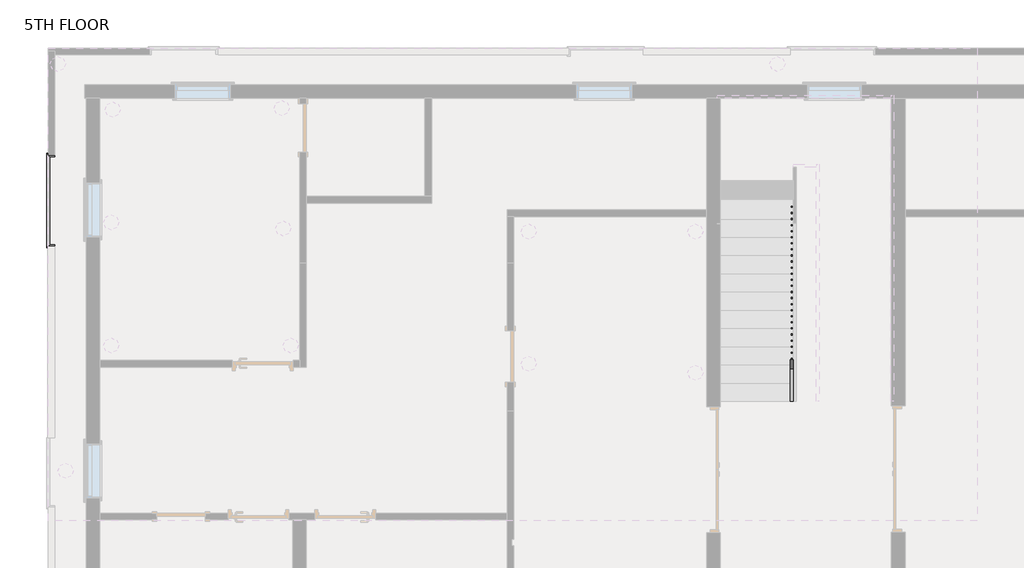
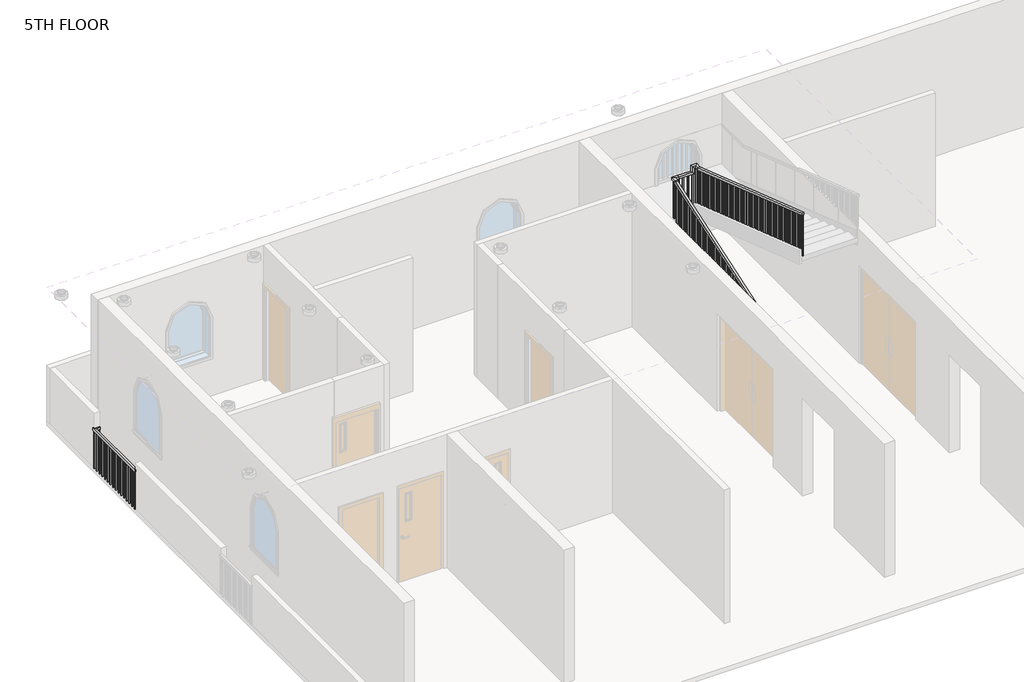
# One storey, part 4 of 7: 2 railings.
"""IFC4 building model written with IfcOpenShell, lengths in millimetres."""

from ifc_helpers import new_model, si_unit, frame, origin, place, context, project, spatial, polyline, outline, extrude, faceted_brep, element, save

model = new_model("IFC4")

# Units and contexts
model_context = context("Model", 3, world=origin())
ifc_project = project(units=[si_unit("LENGTHUNIT", "METRE", prefix="MILLI")], contexts=[model_context])

# Site, building, storey
site = spatial("IfcSite", under=ifc_project)
building = spatial("IfcBuilding", under=site)
storey = spatial("IfcBuildingStorey", under=building, Name="5TH FLOOR", Elevation=16002.0)

# Railings
placement = place(None, origin())
element("IfcRailing", 1, ObjectType="Handrail - Rectangular", at=placement, inside=storey, context=model_context, shape_type="SolidModel", body=[
    faceted_brep([(-680.3987998, 2564.5067329, 17019.8142857), (-680.3987998, 2564.5067329, 16966.1699957), (-629.5987998, 2564.5067329, 16966.1699957), (-629.5987998, 2564.5067329, 17019.8142857), (-680.3987998, 6450.7067329, 18338.3464286), (-680.3987998, 6501.5067329, 18301.9378529), (-629.5987998, 6501.5067329, 18301.9378529), (-629.5987998, 6450.7067329, 18338.3464286), (-553.3987998, 6577.7067329, 18313.4), (-553.3987998, 6577.7067329, 18364.2), (-273.9987915, 6577.7067329, 18364.2), (-223.1987915, 6577.7067329, 18313.4), (-553.3987998, 6526.9067329, 18313.4), (-223.1987915, 6526.9067329, 18313.4), (-553.3987998, 6526.9067329, 18364.2), (-273.9987915, 6526.9067329, 18364.2), (-146.9987915, 2564.5067329, 19812.0), (-197.7987915, 2564.5067329, 19812.0), (-197.7987915, 2564.5067329, 19758.35571), (-146.9987915, 2564.5067329, 19758.35571), (-146.9987915, 6442.3235624, 18442.6678571), (-146.9987915, 6450.7067329, 18493.4678571), (-197.7987915, 6442.3235624, 18442.6678571), (-197.7987915, 6450.7067329, 18493.4678571), (-680.3987998, 6450.7067329, 18364.2), (-680.3987998, 6501.5067329, 18313.4), (-629.5987998, 6501.5067329, 18313.4), (-629.5987998, 6450.7067329, 18364.2), (-680.3987998, 6577.7067329, 18364.2), (-680.3987998, 6577.7067329, 18313.4), (-629.5987998, 6526.9067329, 18313.4), (-629.5987998, 6526.9067329, 18364.2), (-273.9987915, 6577.7067329, 18493.4678571), (-223.1987915, 6577.7067329, 18442.6678571), (-223.1987915, 6526.9067329, 18442.6678571), (-273.9987915, 6526.9067329, 18493.4678571), (-146.9987915, 6577.7067329, 18493.4678571), (-146.9987915, 6577.7067329, 18442.6678571), (-197.7987915, 6526.9067329, 18442.6678571), (-197.7987915, 6526.9067329, 18493.4678571)], [[[0, 1, 2, 3]], [[1, 0, 4, 5]], [[2, 1, 5, 6]], [[3, 2, 6, 7]], [[0, 3, 7, 4]], [[8, 9, 10, 11]], [[12, 8, 11, 13]], [[14, 12, 13, 15]], [[9, 14, 15, 10]], [[16, 17, 18, 19]], [[20, 21, 16, 19]], [[22, 20, 19, 18]], [[23, 22, 18, 17]], [[21, 23, 17, 16]], [[5, 4, 24, 25]], [[6, 5, 25, 26]], [[7, 6, 26, 27]], [[4, 7, 27, 24]], [[25, 24, 28, 29]], [[26, 25, 29, 30]], [[27, 26, 30, 31]], [[24, 27, 31, 28]], [[29, 28, 9, 8]], [[30, 29, 8, 12]], [[31, 30, 12, 14]], [[28, 31, 14, 9]], [[11, 10, 32, 33]], [[13, 11, 33, 34]], [[15, 13, 34, 35]], [[10, 15, 35, 32]], [[33, 32, 36, 37]], [[34, 33, 37, 38]], [[35, 34, 38, 39]], [[32, 35, 39, 36]], [[37, 36, 21, 20]], [[38, 37, 20, 22]], [[39, 38, 22, 23]], [[36, 39, 23, 21]]]),
    extrude(outline(polyline([(2580.3817329, 19752.9695493), (2599.4317329, 19746.5061565), (2599.4317329, 18794.1857143), (2580.3817329, 18794.1857143), (2580.3817329, 19752.9695493)])), frame((-181.9237915, 0.0, 0.0), z_axis=(1.0, 0.0, 0.0), x_axis=(0.0, 1.0, 0.0)), (0.0, 0.0, 1.0), 19.05),
    extrude(outline(polyline([(2681.9817329, 19718.4981207), (2701.0317329, 19712.0347279), (2701.0317329, 18794.1857143), (2681.9817329, 18794.1857143), (2681.9817329, 19718.4981207)])), frame((-181.9237915, 0.0, 0.0), z_axis=(1.0, 0.0, 0.0), x_axis=(0.0, 1.0, 0.0)), (0.0, 0.0, 1.0), 19.05),
    extrude(outline(polyline([(2783.5817329, 19684.0266922), (2802.6317329, 19677.5632993), (2802.6317329, 18794.1857143), (2783.5817329, 18794.1857143), (2783.5817329, 19684.0266922)])), frame((-181.9237915, 0.0, 0.0), z_axis=(1.0, 0.0, 0.0), x_axis=(0.0, 1.0, 0.0)), (0.0, 0.0, 1.0), 19.05),
    extrude(outline(polyline([(2885.1817329, 19649.5552636), (2904.2317329, 19643.0918707), (2904.2317329, 18690.7714286), (2885.1817329, 18690.7714286), (2885.1817329, 19649.5552636)])), frame((-181.9237915, 0.0, 0.0), z_axis=(1.0, 0.0, 0.0), x_axis=(0.0, 1.0, 0.0)), (0.0, 0.0, 1.0), 19.05),
    extrude(outline(polyline([(2986.7817329, 19615.083835), (3005.8317329, 19608.6204422), (3005.8317329, 18690.7714286), (2986.7817329, 18690.7714286), (2986.7817329, 19615.083835)])), frame((-181.9237915, 0.0, 0.0), z_axis=(1.0, 0.0, 0.0), x_axis=(0.0, 1.0, 0.0)), (0.0, 0.0, 1.0), 19.05),
    extrude(outline(polyline([(3088.3817329, 19580.6124065), (3107.4317329, 19574.1490136), (3107.4317329, 18690.7714286), (3088.3817329, 18690.7714286), (3088.3817329, 19580.6124065)])), frame((-181.9237915, 0.0, 0.0), z_axis=(1.0, 0.0, 0.0), x_axis=(0.0, 1.0, 0.0)), (0.0, 0.0, 1.0), 19.05),
    extrude(outline(polyline([(3189.9817329, 19546.1409779), (3209.0317329, 19539.677585), (3209.0317329, 18587.3571429), (3189.9817329, 18587.3571429), (3189.9817329, 19546.1409779)])), frame((-181.9237915, 0.0, 0.0), z_axis=(1.0, 0.0, 0.0), x_axis=(0.0, 1.0, 0.0)), (0.0, 0.0, 1.0), 19.05),
    extrude(outline(polyline([(3291.5817329, 19511.6695493), (3310.6317329, 19505.2061565), (3310.6317329, 18587.3571429), (3291.5817329, 18587.3571429), (3291.5817329, 19511.6695493)])), frame((-181.9237915, 0.0, 0.0), z_axis=(1.0, 0.0, 0.0), x_axis=(0.0, 1.0, 0.0)), (0.0, 0.0, 1.0), 19.05),
    extrude(outline(polyline([(3393.1817329, 19477.1981207), (3412.2317329, 19470.7347279), (3412.2317329, 18587.3571429), (3393.1817329, 18587.3571429), (3393.1817329, 19477.1981207)])), frame((-181.9237915, 0.0, 0.0), z_axis=(1.0, 0.0, 0.0), x_axis=(0.0, 1.0, 0.0)), (0.0, 0.0, 1.0), 19.05),
    extrude(outline(polyline([(3494.7817329, 19442.7266922), (3513.8317329, 19436.2632993), (3513.8317329, 18483.9428571), (3494.7817329, 18483.9428571), (3494.7817329, 19442.7266922)])), frame((-181.9237915, 0.0, 0.0), z_axis=(1.0, 0.0, 0.0), x_axis=(0.0, 1.0, 0.0)), (0.0, 0.0, 1.0), 19.05),
    extrude(outline(polyline([(3596.3817329, 19408.2552636), (3615.4317329, 19401.7918707), (3615.4317329, 18483.9428571), (3596.3817329, 18483.9428571), (3596.3817329, 19408.2552636)])), frame((-181.9237915, 0.0, 0.0), z_axis=(1.0, 0.0, 0.0), x_axis=(0.0, 1.0, 0.0)), (0.0, 0.0, 1.0), 19.05),
    extrude(outline(polyline([(3697.9817329, 19373.783835), (3717.0317329, 19367.3204422), (3717.0317329, 18483.9428571), (3697.9817329, 18483.9428571), (3697.9817329, 19373.783835)])), frame((-181.9237915, 0.0, 0.0), z_axis=(1.0, 0.0, 0.0), x_axis=(0.0, 1.0, 0.0)), (0.0, 0.0, 1.0), 19.05),
    extrude(outline(polyline([(3799.5817329, 19339.3124065), (3818.6317329, 19332.8490136), (3818.6317329, 18380.5285714), (3799.5817329, 18380.5285714), (3799.5817329, 19339.3124065)])), frame((-181.9237915, 0.0, 0.0), z_axis=(1.0, 0.0, 0.0), x_axis=(0.0, 1.0, 0.0)), (0.0, 0.0, 1.0), 19.05),
    extrude(outline(polyline([(3901.1817329, 19304.8409779), (3920.2317329, 19298.377585), (3920.2317329, 18380.5285714), (3901.1817329, 18380.5285714), (3901.1817329, 19304.8409779)])), frame((-181.9237915, 0.0, 0.0), z_axis=(1.0, 0.0, 0.0), x_axis=(0.0, 1.0, 0.0)), (0.0, 0.0, 1.0), 19.05),
    extrude(outline(polyline([(4002.7817329, 19270.3695493), (4021.8317329, 19263.9061565), (4021.8317329, 18380.5285714), (4002.7817329, 18380.5285714), (4002.7817329, 19270.3695493)])), frame((-181.9237915, 0.0, 0.0), z_axis=(1.0, 0.0, 0.0), x_axis=(0.0, 1.0, 0.0)), (0.0, 0.0, 1.0), 19.05),
    extrude(outline(polyline([(4104.3817329, 19235.8981207), (4123.4317329, 19229.4347279), (4123.4317329, 18277.1142857), (4104.3817329, 18277.1142857), (4104.3817329, 19235.8981207)])), frame((-181.9237915, 0.0, 0.0), z_axis=(1.0, 0.0, 0.0), x_axis=(0.0, 1.0, 0.0)), (0.0, 0.0, 1.0), 19.05),
    extrude(outline(polyline([(4205.9817329, 19201.4266922), (4225.0317329, 19194.9632993), (4225.0317329, 18277.1142857), (4205.9817329, 18277.1142857), (4205.9817329, 19201.4266922)])), frame((-181.9237915, 0.0, 0.0), z_axis=(1.0, 0.0, 0.0), x_axis=(0.0, 1.0, 0.0)), (0.0, 0.0, 1.0), 19.05),
    extrude(outline(polyline([(4307.5817329, 19166.9552636), (4326.6317329, 19160.4918707), (4326.6317329, 18277.1142857), (4307.5817329, 18277.1142857), (4307.5817329, 19166.9552636)])), frame((-181.9237915, 0.0, 0.0), z_axis=(1.0, 0.0, 0.0), x_axis=(0.0, 1.0, 0.0)), (0.0, 0.0, 1.0), 19.05),
    extrude(outline(polyline([(4409.1817329, 19132.483835), (4428.2317329, 19126.0204422), (4428.2317329, 18173.7), (4409.1817329, 18173.7), (4409.1817329, 19132.483835)])), frame((-181.9237915, 0.0, 0.0), z_axis=(1.0, 0.0, 0.0), x_axis=(0.0, 1.0, 0.0)), (0.0, 0.0, 1.0), 19.05),
    extrude(outline(polyline([(4510.7817329, 19098.0124065), (4529.8317329, 19091.5490136), (4529.8317329, 18173.7), (4510.7817329, 18173.7), (4510.7817329, 19098.0124065)])), frame((-181.9237915, 0.0, 0.0), z_axis=(1.0, 0.0, 0.0), x_axis=(0.0, 1.0, 0.0)), (0.0, 0.0, 1.0), 19.05),
    extrude(outline(polyline([(4612.3817329, 19063.5409779), (4631.4317329, 19057.077585), (4631.4317329, 18173.7), (4612.3817329, 18173.7), (4612.3817329, 19063.5409779)])), frame((-181.9237915, 0.0, 0.0), z_axis=(1.0, 0.0, 0.0), x_axis=(0.0, 1.0, 0.0)), (0.0, 0.0, 1.0), 19.05),
    extrude(outline(polyline([(4713.9817329, 19029.0695493), (4733.0317329, 19022.6061565), (4733.0317329, 18070.2857143), (4713.9817329, 18070.2857143), (4713.9817329, 19029.0695493)])), frame((-181.9237915, 0.0, 0.0), z_axis=(1.0, 0.0, 0.0), x_axis=(0.0, 1.0, 0.0)), (0.0, 0.0, 1.0), 19.05),
    extrude(outline(polyline([(4815.5817329, 18994.5981207), (4834.6317329, 18988.1347279), (4834.6317329, 18070.2857143), (4815.5817329, 18070.2857143), (4815.5817329, 18994.5981207)])), frame((-181.9237915, 0.0, 0.0), z_axis=(1.0, 0.0, 0.0), x_axis=(0.0, 1.0, 0.0)), (0.0, 0.0, 1.0), 19.05),
    extrude(outline(polyline([(4917.1817329, 18960.1266922), (4936.2317329, 18953.6632993), (4936.2317329, 18070.2857143), (4917.1817329, 18070.2857143), (4917.1817329, 18960.1266922)])), frame((-181.9237915, 0.0, 0.0), z_axis=(1.0, 0.0, 0.0), x_axis=(0.0, 1.0, 0.0)), (0.0, 0.0, 1.0), 19.05),
    extrude(outline(polyline([(5018.7817329, 18925.6552636), (5037.8317329, 18919.1918707), (5037.8317329, 17966.8714286), (5018.7817329, 17966.8714286), (5018.7817329, 18925.6552636)])), frame((-181.9237915, 0.0, 0.0), z_axis=(1.0, 0.0, 0.0), x_axis=(0.0, 1.0, 0.0)), (0.0, 0.0, 1.0), 19.05),
    extrude(outline(polyline([(5120.3817329, 18891.183835), (5139.4317329, 18884.7204422), (5139.4317329, 17966.8714286), (5120.3817329, 17966.8714286), (5120.3817329, 18891.183835)])), frame((-181.9237915, 0.0, 0.0), z_axis=(1.0, 0.0, 0.0), x_axis=(0.0, 1.0, 0.0)), (0.0, 0.0, 1.0), 19.05),
    extrude(outline(polyline([(5221.9817329, 18856.7124065), (5241.0317329, 18850.2490136), (5241.0317329, 17966.8714286), (5221.9817329, 17966.8714286), (5221.9817329, 18856.7124065)])), frame((-181.9237915, 0.0, 0.0), z_axis=(1.0, 0.0, 0.0), x_axis=(0.0, 1.0, 0.0)), (0.0, 0.0, 1.0), 19.05),
    extrude(outline(polyline([(5323.5817329, 18822.2409779), (5342.6317329, 18815.777585), (5342.6317329, 17863.4571429), (5323.5817329, 17863.4571429), (5323.5817329, 18822.2409779)])), frame((-181.9237915, 0.0, 0.0), z_axis=(1.0, 0.0, 0.0), x_axis=(0.0, 1.0, 0.0)), (0.0, 0.0, 1.0), 19.05),
    extrude(outline(polyline([(5425.1817329, 18787.7695493), (5444.2317329, 18781.3061565), (5444.2317329, 17863.4571429), (5425.1817329, 17863.4571429), (5425.1817329, 18787.7695493)])), frame((-181.9237915, 0.0, 0.0), z_axis=(1.0, 0.0, 0.0), x_axis=(0.0, 1.0, 0.0)), (0.0, 0.0, 1.0), 19.05),
    extrude(outline(polyline([(5526.7817329, 18753.2981207), (5545.8317329, 18746.8347279), (5545.8317329, 17863.4571429), (5526.7817329, 17863.4571429), (5526.7817329, 18753.2981207)])), frame((-181.9237915, 0.0, 0.0), z_axis=(1.0, 0.0, 0.0), x_axis=(0.0, 1.0, 0.0)), (0.0, 0.0, 1.0), 19.05),
    extrude(outline(polyline([(5628.3817329, 18718.8266922), (5647.4317329, 18712.3632993), (5647.4317329, 17760.0428571), (5628.3817329, 17760.0428571), (5628.3817329, 18718.8266922)])), frame((-181.9237915, 0.0, 0.0), z_axis=(1.0, 0.0, 0.0), x_axis=(0.0, 1.0, 0.0)), (0.0, 0.0, 1.0), 19.05),
    extrude(outline(polyline([(5729.9817329, 18684.3552636), (5749.0317329, 18677.8918707), (5749.0317329, 17760.0428571), (5729.9817329, 17760.0428571), (5729.9817329, 18684.3552636)])), frame((-181.9237915, 0.0, 0.0), z_axis=(1.0, 0.0, 0.0), x_axis=(0.0, 1.0, 0.0)), (0.0, 0.0, 1.0), 19.05),
    extrude(outline(polyline([(5831.5817329, 18649.883835), (5850.6317329, 18643.4204422), (5850.6317329, 17760.0428571), (5831.5817329, 17760.0428571), (5831.5817329, 18649.883835)])), frame((-181.9237915, 0.0, 0.0), z_axis=(1.0, 0.0, 0.0), x_axis=(0.0, 1.0, 0.0)), (0.0, 0.0, 1.0), 19.05),
    extrude(outline(polyline([(5933.1817329, 18615.4124065), (5952.2317329, 18608.9490136), (5952.2317329, 17656.6285714), (5933.1817329, 17656.6285714), (5933.1817329, 18615.4124065)])), frame((-181.9237915, 0.0, 0.0), z_axis=(1.0, 0.0, 0.0), x_axis=(0.0, 1.0, 0.0)), (0.0, 0.0, 1.0), 19.05),
    extrude(outline(polyline([(6034.7817329, 18580.9409779), (6053.8317329, 18574.477585), (6053.8317329, 17656.6285714), (6034.7817329, 17656.6285714), (6034.7817329, 18580.9409779)])), frame((-181.9237915, 0.0, 0.0), z_axis=(1.0, 0.0, 0.0), x_axis=(0.0, 1.0, 0.0)), (0.0, 0.0, 1.0), 19.05),
    extrude(outline(polyline([(6136.3817329, 18546.4695493), (6155.4317329, 18540.0061565), (6155.4317329, 17656.6285714), (6136.3817329, 17656.6285714), (6136.3817329, 18546.4695493)])), frame((-181.9237915, 0.0, 0.0), z_axis=(1.0, 0.0, 0.0), x_axis=(0.0, 1.0, 0.0)), (0.0, 0.0, 1.0), 19.05),
    extrude(outline(polyline([(6237.9817329, 18511.9981207), (6257.0317329, 18505.5347279), (6257.0317329, 17553.2142857), (6237.9817329, 17553.2142857), (6237.9817329, 18511.9981207)])), frame((-181.9237915, 0.0, 0.0), z_axis=(1.0, 0.0, 0.0), x_axis=(0.0, 1.0, 0.0)), (0.0, 0.0, 1.0), 19.05),
    extrude(outline(polyline([(6339.5817329, 18477.5266922), (6358.6317329, 18471.0632993), (6358.6317329, 17553.2142857), (6339.5817329, 17553.2142857), (6339.5817329, 18477.5266922)])), frame((-181.9237915, 0.0, 0.0), z_axis=(1.0, 0.0, 0.0), x_axis=(0.0, 1.0, 0.0)), (0.0, 0.0, 1.0), 19.05),
    extrude(outline(polyline([(6441.1817329, 18443.0552636), (6460.2317329, 18436.5918707), (6460.2317329, 17553.2142857), (6441.1817329, 17553.2142857), (6441.1817329, 18443.0552636)])), frame((-181.9237915, 0.0, 0.0), z_axis=(1.0, 0.0, 0.0), x_axis=(0.0, 1.0, 0.0)), (0.0, 0.0, 1.0), 19.05),
    extrude(outline(polyline([(-258.1237998, 6542.7817329), (-258.1237998, 6561.8317329), (-239.0737998, 6561.8317329), (-239.0737998, 6542.7817329), (-258.1237998, 6542.7817329)])), frame((0.0, 0.0, 17449.8), z_axis=(0.0, 0.0, 1.0), x_axis=(1.0, 0.0, 0.0)), (0.0, 0.0, 1.0), 992.8678571),
    extrude(outline(polyline([(-359.7237998, 6542.7817329), (-359.7237998, 6561.8317329), (-340.6737998, 6561.8317329), (-340.6737998, 6542.7817329), (-359.7237998, 6542.7817329)])), frame((0.0, 0.0, 17449.8), z_axis=(0.0, 0.0, 1.0), x_axis=(1.0, 0.0, 0.0)), (0.0, 0.0, 1.0), 863.6),
    extrude(outline(polyline([(-461.3237998, 6542.7817329), (-461.3237998, 6561.8317329), (-442.2737998, 6561.8317329), (-442.2737998, 6542.7817329), (-461.3237998, 6542.7817329)])), frame((0.0, 0.0, 17449.8), z_axis=(0.0, 0.0, 1.0), x_axis=(1.0, 0.0, 0.0)), (0.0, 0.0, 1.0), 863.6),
    extrude(outline(polyline([(-562.9237998, 6542.7817329), (-562.9237998, 6561.8317329), (-543.8737998, 6561.8317329), (-543.8737998, 6542.7817329), (-562.9237998, 6542.7817329)])), frame((0.0, 0.0, 17449.8), z_axis=(0.0, 0.0, 1.0), x_axis=(1.0, 0.0, 0.0)), (0.0, 0.0, 1.0), 863.6),
    extrude(outline(polyline([(-645.4737998, 6517.3817329), (-664.5237998, 6517.3817329), (-664.5237998, 6536.4317329), (-645.4737998, 6536.4317329), (-645.4737998, 6517.3817329)])), frame((0.0, 0.0, 17449.8), z_axis=(0.0, 0.0, 1.0), x_axis=(1.0, 0.0, 0.0)), (0.0, 0.0, 1.0), 863.6),
    extrude(outline(polyline([(6415.7817329, 18272.852585), (6434.8317329, 18279.3159779), (6434.8317329, 17346.3857143), (6415.7817329, 17346.3857143), (6415.7817329, 18272.852585)])), frame((-664.5237998, 0.0, 0.0), z_axis=(1.0, 0.0, 0.0), x_axis=(0.0, 1.0, 0.0)), (0.0, 0.0, 1.0), 19.05),
    extrude(outline(polyline([(6314.1817329, 18238.3811565), (6333.2317329, 18244.8445493), (6333.2317329, 17346.3857143), (6314.1817329, 17346.3857143), (6314.1817329, 18238.3811565)])), frame((-664.5237998, 0.0, 0.0), z_axis=(1.0, 0.0, 0.0), x_axis=(0.0, 1.0, 0.0)), (0.0, 0.0, 1.0), 19.05),
    extrude(outline(polyline([(6212.5817329, 18203.9097279), (6231.6317329, 18210.3731207), (6231.6317329, 17346.3857143), (6212.5817329, 17346.3857143), (6212.5817329, 18203.9097279)])), frame((-664.5237998, 0.0, 0.0), z_axis=(1.0, 0.0, 0.0), x_axis=(0.0, 1.0, 0.0)), (0.0, 0.0, 1.0), 19.05),
    extrude(outline(polyline([(6110.9817329, 18169.4382993), (6130.0317329, 18175.9016922), (6130.0317329, 17242.9714286), (6110.9817329, 17242.9714286), (6110.9817329, 18169.4382993)])), frame((-664.5237998, 0.0, 0.0), z_axis=(1.0, 0.0, 0.0), x_axis=(0.0, 1.0, 0.0)), (0.0, 0.0, 1.0), 19.05),
    extrude(outline(polyline([(6009.3817329, 18134.9668707), (6028.4317329, 18141.4302636), (6028.4317329, 17242.9714286), (6009.3817329, 17242.9714286), (6009.3817329, 18134.9668707)])), frame((-664.5237998, 0.0, 0.0), z_axis=(1.0, 0.0, 0.0), x_axis=(0.0, 1.0, 0.0)), (0.0, 0.0, 1.0), 19.05),
    extrude(outline(polyline([(5907.7817329, 18100.4954422), (5926.8317329, 18106.958835), (5926.8317329, 17242.9714286), (5907.7817329, 17242.9714286), (5907.7817329, 18100.4954422)])), frame((-664.5237998, 0.0, 0.0), z_axis=(1.0, 0.0, 0.0), x_axis=(0.0, 1.0, 0.0)), (0.0, 0.0, 1.0), 19.05),
    extrude(outline(polyline([(5806.1817329, 18066.0240136), (5825.2317329, 18072.4874065), (5825.2317329, 17139.5571429), (5806.1817329, 17139.5571429), (5806.1817329, 18066.0240136)])), frame((-664.5237998, 0.0, 0.0), z_axis=(1.0, 0.0, 0.0), x_axis=(0.0, 1.0, 0.0)), (0.0, 0.0, 1.0), 19.05),
    extrude(outline(polyline([(5704.5817329, 18031.552585), (5723.6317329, 18038.0159779), (5723.6317329, 17139.5571429), (5704.5817329, 17139.5571429), (5704.5817329, 18031.552585)])), frame((-664.5237998, 0.0, 0.0), z_axis=(1.0, 0.0, 0.0), x_axis=(0.0, 1.0, 0.0)), (0.0, 0.0, 1.0), 19.05),
    extrude(outline(polyline([(5602.9817329, 17997.0811565), (5622.0317329, 18003.5445493), (5622.0317329, 17139.5571429), (5602.9817329, 17139.5571429), (5602.9817329, 17997.0811565)])), frame((-664.5237998, 0.0, 0.0), z_axis=(1.0, 0.0, 0.0), x_axis=(0.0, 1.0, 0.0)), (0.0, 0.0, 1.0), 19.05),
    extrude(outline(polyline([(5501.3817329, 17962.6097279), (5520.4317329, 17969.0731207), (5520.4317329, 17036.1428571), (5501.3817329, 17036.1428571), (5501.3817329, 17962.6097279)])), frame((-664.5237998, 0.0, 0.0), z_axis=(1.0, 0.0, 0.0), x_axis=(0.0, 1.0, 0.0)), (0.0, 0.0, 1.0), 19.05),
    extrude(outline(polyline([(5399.7817329, 17928.1382993), (5418.8317329, 17934.6016922), (5418.8317329, 17036.1428571), (5399.7817329, 17036.1428571), (5399.7817329, 17928.1382993)])), frame((-664.5237998, 0.0, 0.0), z_axis=(1.0, 0.0, 0.0), x_axis=(0.0, 1.0, 0.0)), (0.0, 0.0, 1.0), 19.05),
    extrude(outline(polyline([(5298.1817329, 17893.6668707), (5317.2317329, 17900.1302636), (5317.2317329, 17036.1428571), (5298.1817329, 17036.1428571), (5298.1817329, 17893.6668707)])), frame((-664.5237998, 0.0, 0.0), z_axis=(1.0, 0.0, 0.0), x_axis=(0.0, 1.0, 0.0)), (0.0, 0.0, 1.0), 19.05),
    extrude(outline(polyline([(5196.5817329, 17859.1954422), (5215.6317329, 17865.658835), (5215.6317329, 16932.7285714), (5196.5817329, 16932.7285714), (5196.5817329, 17859.1954422)])), frame((-664.5237998, 0.0, 0.0), z_axis=(1.0, 0.0, 0.0), x_axis=(0.0, 1.0, 0.0)), (0.0, 0.0, 1.0), 19.05),
    extrude(outline(polyline([(5094.9817329, 17824.7240136), (5114.0317329, 17831.1874065), (5114.0317329, 16932.7285714), (5094.9817329, 16932.7285714), (5094.9817329, 17824.7240136)])), frame((-664.5237998, 0.0, 0.0), z_axis=(1.0, 0.0, 0.0), x_axis=(0.0, 1.0, 0.0)), (0.0, 0.0, 1.0), 19.05),
    extrude(outline(polyline([(4993.3817329, 17790.252585), (5012.4317329, 17796.7159779), (5012.4317329, 16932.7285714), (4993.3817329, 16932.7285714), (4993.3817329, 17790.252585)])), frame((-664.5237998, 0.0, 0.0), z_axis=(1.0, 0.0, 0.0), x_axis=(0.0, 1.0, 0.0)), (0.0, 0.0, 1.0), 19.05),
    extrude(outline(polyline([(4891.7817329, 17755.7811565), (4910.8317329, 17762.2445493), (4910.8317329, 16829.3142857), (4891.7817329, 16829.3142857), (4891.7817329, 17755.7811565)])), frame((-664.5237998, 0.0, 0.0), z_axis=(1.0, 0.0, 0.0), x_axis=(0.0, 1.0, 0.0)), (0.0, 0.0, 1.0), 19.05),
    extrude(outline(polyline([(4790.1817329, 17721.3097279), (4809.2317329, 17727.7731207), (4809.2317329, 16829.3142857), (4790.1817329, 16829.3142857), (4790.1817329, 17721.3097279)])), frame((-664.5237998, 0.0, 0.0), z_axis=(1.0, 0.0, 0.0), x_axis=(0.0, 1.0, 0.0)), (0.0, 0.0, 1.0), 19.05),
    extrude(outline(polyline([(4688.5817329, 17686.8382993), (4707.6317329, 17693.3016922), (4707.6317329, 16829.3142857), (4688.5817329, 16829.3142857), (4688.5817329, 17686.8382993)])), frame((-664.5237998, 0.0, 0.0), z_axis=(1.0, 0.0, 0.0), x_axis=(0.0, 1.0, 0.0)), (0.0, 0.0, 1.0), 19.05),
    extrude(outline(polyline([(4586.9817329, 17652.3668707), (4606.0317329, 17658.8302636), (4606.0317329, 16725.9), (4586.9817329, 16725.9), (4586.9817329, 17652.3668707)])), frame((-664.5237998, 0.0, 0.0), z_axis=(1.0, 0.0, 0.0), x_axis=(0.0, 1.0, 0.0)), (0.0, 0.0, 1.0), 19.05),
    extrude(outline(polyline([(4485.3817329, 17617.8954422), (4504.4317329, 17624.358835), (4504.4317329, 16725.9), (4485.3817329, 16725.9), (4485.3817329, 17617.8954422)])), frame((-664.5237998, 0.0, 0.0), z_axis=(1.0, 0.0, 0.0), x_axis=(0.0, 1.0, 0.0)), (0.0, 0.0, 1.0), 19.05),
    extrude(outline(polyline([(4383.7817329, 17583.4240136), (4402.8317329, 17589.8874065), (4402.8317329, 16725.9), (4383.7817329, 16725.9), (4383.7817329, 17583.4240136)])), frame((-664.5237998, 0.0, 0.0), z_axis=(1.0, 0.0, 0.0), x_axis=(0.0, 1.0, 0.0)), (0.0, 0.0, 1.0), 19.05),
    extrude(outline(polyline([(4282.1817329, 17548.952585), (4301.2317329, 17555.4159779), (4301.2317329, 16622.4857143), (4282.1817329, 16622.4857143), (4282.1817329, 17548.952585)])), frame((-664.5237998, 0.0, 0.0), z_axis=(1.0, 0.0, 0.0), x_axis=(0.0, 1.0, 0.0)), (0.0, 0.0, 1.0), 19.05),
    extrude(outline(polyline([(4180.5817329, 17514.4811565), (4199.6317329, 17520.9445493), (4199.6317329, 16622.4857143), (4180.5817329, 16622.4857143), (4180.5817329, 17514.4811565)])), frame((-664.5237998, 0.0, 0.0), z_axis=(1.0, 0.0, 0.0), x_axis=(0.0, 1.0, 0.0)), (0.0, 0.0, 1.0), 19.05),
    extrude(outline(polyline([(4078.9817329, 17480.0097279), (4098.0317329, 17486.4731207), (4098.0317329, 16622.4857143), (4078.9817329, 16622.4857143), (4078.9817329, 17480.0097279)])), frame((-664.5237998, 0.0, 0.0), z_axis=(1.0, 0.0, 0.0), x_axis=(0.0, 1.0, 0.0)), (0.0, 0.0, 1.0), 19.05),
    extrude(outline(polyline([(3977.3817329, 17445.5382993), (3996.4317329, 17452.0016922), (3996.4317329, 16519.0714286), (3977.3817329, 16519.0714286), (3977.3817329, 17445.5382993)])), frame((-664.5237998, 0.0, 0.0), z_axis=(1.0, 0.0, 0.0), x_axis=(0.0, 1.0, 0.0)), (0.0, 0.0, 1.0), 19.05),
    extrude(outline(polyline([(3875.7817329, 17411.0668707), (3894.8317329, 17417.5302636), (3894.8317329, 16519.0714286), (3875.7817329, 16519.0714286), (3875.7817329, 17411.0668707)])), frame((-664.5237998, 0.0, 0.0), z_axis=(1.0, 0.0, 0.0), x_axis=(0.0, 1.0, 0.0)), (0.0, 0.0, 1.0), 19.05),
    extrude(outline(polyline([(3774.1817329, 17376.5954422), (3793.2317329, 17383.058835), (3793.2317329, 16519.0714286), (3774.1817329, 16519.0714286), (3774.1817329, 17376.5954422)])), frame((-664.5237998, 0.0, 0.0), z_axis=(1.0, 0.0, 0.0), x_axis=(0.0, 1.0, 0.0)), (0.0, 0.0, 1.0), 19.05),
    extrude(outline(polyline([(3672.5817329, 17342.1240136), (3691.6317329, 17348.5874065), (3691.6317329, 16415.6571429), (3672.5817329, 16415.6571429), (3672.5817329, 17342.1240136)])), frame((-664.5237998, 0.0, 0.0), z_axis=(1.0, 0.0, 0.0), x_axis=(0.0, 1.0, 0.0)), (0.0, 0.0, 1.0), 19.05),
    extrude(outline(polyline([(3570.9817329, 17307.652585), (3590.0317329, 17314.1159779), (3590.0317329, 16415.6571429), (3570.9817329, 16415.6571429), (3570.9817329, 17307.652585)])), frame((-664.5237998, 0.0, 0.0), z_axis=(1.0, 0.0, 0.0), x_axis=(0.0, 1.0, 0.0)), (0.0, 0.0, 1.0), 19.05),
    extrude(outline(polyline([(3469.3817329, 17273.1811565), (3488.4317329, 17279.6445493), (3488.4317329, 16415.6571429), (3469.3817329, 16415.6571429), (3469.3817329, 17273.1811565)])), frame((-664.5237998, 0.0, 0.0), z_axis=(1.0, 0.0, 0.0), x_axis=(0.0, 1.0, 0.0)), (0.0, 0.0, 1.0), 19.05),
    extrude(outline(polyline([(3367.7817329, 17238.7097279), (3386.8317329, 17245.1731207), (3386.8317329, 16312.2428571), (3367.7817329, 16312.2428571), (3367.7817329, 17238.7097279)])), frame((-664.5237998, 0.0, 0.0), z_axis=(1.0, 0.0, 0.0), x_axis=(0.0, 1.0, 0.0)), (0.0, 0.0, 1.0), 19.05),
    extrude(outline(polyline([(3266.1817329, 17204.2382993), (3285.2317329, 17210.7016922), (3285.2317329, 16312.2428571), (3266.1817329, 16312.2428571), (3266.1817329, 17204.2382993)])), frame((-664.5237998, 0.0, 0.0), z_axis=(1.0, 0.0, 0.0), x_axis=(0.0, 1.0, 0.0)), (0.0, 0.0, 1.0), 19.05),
    extrude(outline(polyline([(3164.5817329, 17169.7668707), (3183.6317329, 17176.2302636), (3183.6317329, 16312.2428571), (3164.5817329, 16312.2428571), (3164.5817329, 17169.7668707)])), frame((-664.5237998, 0.0, 0.0), z_axis=(1.0, 0.0, 0.0), x_axis=(0.0, 1.0, 0.0)), (0.0, 0.0, 1.0), 19.05),
    extrude(outline(polyline([(3062.9817329, 17135.2954422), (3082.0317329, 17141.758835), (3082.0317329, 16208.8285714), (3062.9817329, 16208.8285714), (3062.9817329, 17135.2954422)])), frame((-664.5237998, 0.0, 0.0), z_axis=(1.0, 0.0, 0.0), x_axis=(0.0, 1.0, 0.0)), (0.0, 0.0, 1.0), 19.05),
    extrude(outline(polyline([(2961.3817329, 17100.8240136), (2980.4317329, 17107.2874065), (2980.4317329, 16208.8285714), (2961.3817329, 16208.8285714), (2961.3817329, 17100.8240136)])), frame((-664.5237998, 0.0, 0.0), z_axis=(1.0, 0.0, 0.0), x_axis=(0.0, 1.0, 0.0)), (0.0, 0.0, 1.0), 19.05),
    extrude(outline(polyline([(2859.7817329, 17066.352585), (2878.8317329, 17072.8159779), (2878.8317329, 16208.8285714), (2859.7817329, 16208.8285714), (2859.7817329, 17066.352585)])), frame((-664.5237998, 0.0, 0.0), z_axis=(1.0, 0.0, 0.0), x_axis=(0.0, 1.0, 0.0)), (0.0, 0.0, 1.0), 19.05),
    extrude(outline(polyline([(2758.1817329, 17031.8811565), (2777.2317329, 17038.3445493), (2777.2317329, 16105.4142857), (2758.1817329, 16105.4142857), (2758.1817329, 17031.8811565)])), frame((-664.5237998, 0.0, 0.0), z_axis=(1.0, 0.0, 0.0), x_axis=(0.0, 1.0, 0.0)), (0.0, 0.0, 1.0), 19.05),
    extrude(outline(polyline([(2656.5817329, 16997.4097279), (2675.6317329, 17003.8731207), (2675.6317329, 16105.4142857), (2656.5817329, 16105.4142857), (2656.5817329, 16997.4097279)])), frame((-664.5237998, 0.0, 0.0), z_axis=(1.0, 0.0, 0.0), x_axis=(0.0, 1.0, 0.0)), (0.0, 0.0, 1.0), 19.05),
    extrude(outline(polyline([(-181.9237915, 6542.7817329), (-181.9237915, 6561.8317329), (-162.8737915, 6561.8317329), (-162.8737915, 6542.7817329), (-181.9237915, 6542.7817329)])), frame((0.0, 0.0, 17449.8), z_axis=(0.0, 0.0, 1.0), x_axis=(1.0, 0.0, 0.0)), (0.0, 0.0, 1.0), 992.8678571),
    extrude(outline(polyline([(-645.4737998, 6542.7817329), (-664.5237998, 6542.7817329), (-664.5237998, 6561.8317329), (-645.4737998, 6561.8317329), (-645.4737998, 6542.7817329)])), frame((0.0, 0.0, 17449.8), z_axis=(0.0, 0.0, 1.0), x_axis=(1.0, 0.0, 0.0)), (0.0, 0.0, 1.0), 863.6),
    extrude(outline(polyline([(2564.5067329, 19758.35571), (2583.5567329, 19751.8923172), (2583.5567329, 18794.1857143), (2564.5067329, 18794.1857143), (2564.5067329, 19758.35571)])), frame((-181.9237915, 0.0, 0.0), z_axis=(1.0, 0.0, 0.0), x_axis=(0.0, 1.0, 0.0)), (0.0, 0.0, 1.0), 19.05),
    extrude(outline(polyline([(2564.5067329, 16966.1699957), (2583.5567329, 16972.6333886), (2583.5567329, 16105.4142857), (2564.5067329, 16105.4142857), (2564.5067329, 16966.1699957)])), frame((-664.5237998, 0.0, 0.0), z_axis=(1.0, 0.0, 0.0), x_axis=(0.0, 1.0, 0.0)), (0.0, 0.0, 1.0), 19.05),
])
element("IfcRailing", 2, ObjectType="Handrail - Rectangular", at=placement, inside=storey, context=model_context, shape_type="SolidModel", body=[
    faceted_brep([(-12973.9987925, 6656.8711337, 16916.4), (-12973.9987925, 6656.8711337, 16865.6), (-12973.9987925, 6707.6711337, 16865.6), (-12973.9987925, 6707.6711337, 16916.4), (-13062.8987925, 6656.8711337, 16916.4), (-13062.8987925, 6656.8711337, 16865.6), (-13113.6987925, 6707.6711337, 16865.6), (-13113.6987925, 6707.6711337, 16916.4), (-13062.8987925, 5180.1736362, 16916.4), (-13062.8987925, 5180.1736362, 16865.6), (-13113.6987925, 5129.3736362, 16865.6), (-13113.6987925, 5129.3736362, 16916.4), (-12973.9987925, 5180.1736362, 16916.4), (-12973.9987925, 5129.3736362, 16916.4), (-12973.9987925, 5129.3736362, 16865.6), (-12973.9987925, 5180.1736362, 16865.6)], [[[0, 1, 2, 3]], [[1, 0, 4, 5]], [[2, 1, 5, 6]], [[3, 2, 6, 7]], [[0, 3, 7, 4]], [[5, 4, 8, 9]], [[6, 5, 9, 10]], [[7, 6, 10, 11]], [[4, 7, 11, 8]], [[12, 13, 14, 15]], [[9, 8, 12, 15]], [[10, 9, 15, 14]], [[11, 10, 14, 13]], [[8, 11, 13, 12]]]),
    extrude(outline(polyline([(-12996.2237925, 5145.2486362), (-12996.2237925, 5164.2986362), (-12977.1737925, 5164.2986362), (-12977.1737925, 5145.2486362), (-12996.2237925, 5145.2486362)])), frame((0.0, 0.0, 16002.0), z_axis=(0.0, 0.0, 1.0), x_axis=(1.0, 0.0, 0.0)), (0.0, 0.0, 1.0), 863.6),
    extrude(outline(polyline([(-13097.8237925, 5167.7961337), (-13078.7737925, 5167.7961337), (-13078.7737925, 5148.7461337), (-13097.8237925, 5148.7461337), (-13097.8237925, 5167.7961337)])), frame((0.0, 0.0, 16002.0), z_axis=(0.0, 0.0, 1.0), x_axis=(1.0, 0.0, 0.0)), (0.0, 0.0, 1.0), 863.6),
    extrude(outline(polyline([(-13097.8237925, 5269.3961337), (-13078.7737925, 5269.3961337), (-13078.7737925, 5250.3461337), (-13097.8237925, 5250.3461337), (-13097.8237925, 5269.3961337)])), frame((0.0, 0.0, 16002.0), z_axis=(0.0, 0.0, 1.0), x_axis=(1.0, 0.0, 0.0)), (0.0, 0.0, 1.0), 863.6),
    extrude(outline(polyline([(-13097.8237925, 5370.9961337), (-13078.7737925, 5370.9961337), (-13078.7737925, 5351.9461337), (-13097.8237925, 5351.9461337), (-13097.8237925, 5370.9961337)])), frame((0.0, 0.0, 16002.0), z_axis=(0.0, 0.0, 1.0), x_axis=(1.0, 0.0, 0.0)), (0.0, 0.0, 1.0), 863.6),
    extrude(outline(polyline([(-13097.8237925, 5472.5961337), (-13078.7737925, 5472.5961337), (-13078.7737925, 5453.5461337), (-13097.8237925, 5453.5461337), (-13097.8237925, 5472.5961337)])), frame((0.0, 0.0, 16002.0), z_axis=(0.0, 0.0, 1.0), x_axis=(1.0, 0.0, 0.0)), (0.0, 0.0, 1.0), 863.6),
    extrude(outline(polyline([(-13097.8237925, 5574.1961337), (-13078.7737925, 5574.1961337), (-13078.7737925, 5555.1461337), (-13097.8237925, 5555.1461337), (-13097.8237925, 5574.1961337)])), frame((0.0, 0.0, 16002.0), z_axis=(0.0, 0.0, 1.0), x_axis=(1.0, 0.0, 0.0)), (0.0, 0.0, 1.0), 863.6),
    extrude(outline(polyline([(-13097.8237925, 5675.7961337), (-13078.7737925, 5675.7961337), (-13078.7737925, 5656.7461337), (-13097.8237925, 5656.7461337), (-13097.8237925, 5675.7961337)])), frame((0.0, 0.0, 16002.0), z_axis=(0.0, 0.0, 1.0), x_axis=(1.0, 0.0, 0.0)), (0.0, 0.0, 1.0), 863.6),
    extrude(outline(polyline([(-13097.8237925, 5777.3961337), (-13078.7737925, 5777.3961337), (-13078.7737925, 5758.3461337), (-13097.8237925, 5758.3461337), (-13097.8237925, 5777.3961337)])), frame((0.0, 0.0, 16002.0), z_axis=(0.0, 0.0, 1.0), x_axis=(1.0, 0.0, 0.0)), (0.0, 0.0, 1.0), 863.6),
    extrude(outline(polyline([(-13097.8237925, 5878.9961337), (-13078.7737925, 5878.9961337), (-13078.7737925, 5859.9461337), (-13097.8237925, 5859.9461337), (-13097.8237925, 5878.9961337)])), frame((0.0, 0.0, 16002.0), z_axis=(0.0, 0.0, 1.0), x_axis=(1.0, 0.0, 0.0)), (0.0, 0.0, 1.0), 863.6),
    extrude(outline(polyline([(-13097.8237925, 5980.5961337), (-13078.7737925, 5980.5961337), (-13078.7737925, 5961.5461337), (-13097.8237925, 5961.5461337), (-13097.8237925, 5980.5961337)])), frame((0.0, 0.0, 16002.0), z_axis=(0.0, 0.0, 1.0), x_axis=(1.0, 0.0, 0.0)), (0.0, 0.0, 1.0), 863.6),
    extrude(outline(polyline([(-13097.8237925, 6082.1961337), (-13078.7737925, 6082.1961337), (-13078.7737925, 6063.1461337), (-13097.8237925, 6063.1461337), (-13097.8237925, 6082.1961337)])), frame((0.0, 0.0, 16002.0), z_axis=(0.0, 0.0, 1.0), x_axis=(1.0, 0.0, 0.0)), (0.0, 0.0, 1.0), 863.6),
    extrude(outline(polyline([(-13097.8237925, 6183.7961337), (-13078.7737925, 6183.7961337), (-13078.7737925, 6164.7461337), (-13097.8237925, 6164.7461337), (-13097.8237925, 6183.7961337)])), frame((0.0, 0.0, 16002.0), z_axis=(0.0, 0.0, 1.0), x_axis=(1.0, 0.0, 0.0)), (0.0, 0.0, 1.0), 863.6),
    extrude(outline(polyline([(-13097.8237925, 6285.3961337), (-13078.7737925, 6285.3961337), (-13078.7737925, 6266.3461337), (-13097.8237925, 6266.3461337), (-13097.8237925, 6285.3961337)])), frame((0.0, 0.0, 16002.0), z_axis=(0.0, 0.0, 1.0), x_axis=(1.0, 0.0, 0.0)), (0.0, 0.0, 1.0), 863.6),
    extrude(outline(polyline([(-13097.8237925, 6386.9961337), (-13078.7737925, 6386.9961337), (-13078.7737925, 6367.9461337), (-13097.8237925, 6367.9461337), (-13097.8237925, 6386.9961337)])), frame((0.0, 0.0, 16002.0), z_axis=(0.0, 0.0, 1.0), x_axis=(1.0, 0.0, 0.0)), (0.0, 0.0, 1.0), 863.6),
    extrude(outline(polyline([(-13097.8237925, 6488.5961337), (-13078.7737925, 6488.5961337), (-13078.7737925, 6469.5461337), (-13097.8237925, 6469.5461337), (-13097.8237925, 6488.5961337)])), frame((0.0, 0.0, 16002.0), z_axis=(0.0, 0.0, 1.0), x_axis=(1.0, 0.0, 0.0)), (0.0, 0.0, 1.0), 863.6),
    extrude(outline(polyline([(-13097.8237925, 6590.1961337), (-13078.7737925, 6590.1961337), (-13078.7737925, 6571.1461337), (-13097.8237925, 6571.1461337), (-13097.8237925, 6590.1961337)])), frame((0.0, 0.0, 16002.0), z_axis=(0.0, 0.0, 1.0), x_axis=(1.0, 0.0, 0.0)), (0.0, 0.0, 1.0), 863.6),
    extrude(outline(polyline([(-13066.0737925, 6691.7961337), (-13066.0737925, 6672.7461337), (-13085.1237925, 6672.7461337), (-13085.1237925, 6691.7961337), (-13066.0737925, 6691.7961337)])), frame((0.0, 0.0, 16002.0), z_axis=(0.0, 0.0, 1.0), x_axis=(1.0, 0.0, 0.0)), (0.0, 0.0, 1.0), 863.6),
    extrude(outline(polyline([(-13097.8237925, 5164.2986362), (-13078.7737925, 5164.2986362), (-13078.7737925, 5145.2486362), (-13097.8237925, 5145.2486362), (-13097.8237925, 5164.2986362)])), frame((0.0, 0.0, 16002.0), z_axis=(0.0, 0.0, 1.0), x_axis=(1.0, 0.0, 0.0)), (0.0, 0.0, 1.0), 863.6),
    extrude(outline(polyline([(-13078.7737925, 6691.7961337), (-13078.7737925, 6672.7461337), (-13097.8237925, 6672.7461337), (-13097.8237925, 6691.7961337), (-13078.7737925, 6691.7961337)])), frame((0.0, 0.0, 16002.0), z_axis=(0.0, 0.0, 1.0), x_axis=(1.0, 0.0, 0.0)), (0.0, 0.0, 1.0), 863.6),
    extrude(outline(polyline([(-12993.0487925, 5145.2486362), (-12993.0487925, 5164.2986362), (-12973.9987925, 5164.2986362), (-12973.9987925, 5145.2486362), (-12993.0487925, 5145.2486362)])), frame((0.0, 0.0, 16002.0), z_axis=(0.0, 0.0, 1.0), x_axis=(1.0, 0.0, 0.0)), (0.0, 0.0, 1.0), 863.6),
    extrude(outline(polyline([(-12973.9987925, 6691.7961337), (-12973.9987925, 6672.7461337), (-12993.0487925, 6672.7461337), (-12993.0487925, 6691.7961337), (-12973.9987925, 6691.7961337)])), frame((0.0, 0.0, 16002.0), z_axis=(0.0, 0.0, 1.0), x_axis=(1.0, 0.0, 0.0)), (0.0, 0.0, 1.0), 863.6),
])

save(model, "model.ifc")

# Revit data of these elements
# Type "Handrail - Rectangular"
#   Assembly Code = "C2010400"
#   built-in parameter 1008612 = 0.0416667 (stored number, unit not read)
#   built-in parameter 1008611 = 0.0416667 (stored number, unit not read)
#   built-in parameter 1008609 = 0.333333 (stored number, unit not read)
#   built-in parameter 1008604 = 0.166667 (stored number, unit not read)
#   built-in parameter 1008603 = 0.166667 (stored number, unit not read)
#   Railing Height = 3' - 0"
#   built-in parameter 1008630 = 2
#   built-in parameter 1008610 = 2
#   built-in parameter 1008618 = Baluster - Square : 3/4"
# Elements 1, 2 (IfcRailing, "Handrail - Rectangular")
#   Phase Created = New Construction
